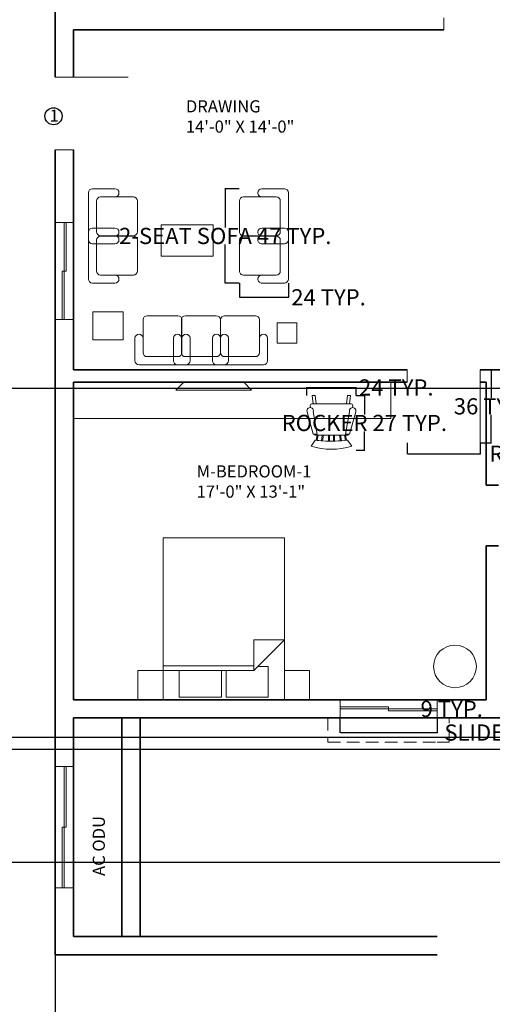
# Model space of a CAD drawing. Units: inches. Extents: x 3343 to 4790, y 1140 to 2641.
# Tile 7 of 10: x 4104 to 4337, y 1710 to 2196. Entities that reach past the tile are written whole.
import ezdxf

# ---------------------------------------------------------------- set-up
doc = ezdxf.new("R2010")
doc.units = ezdxf.units.IN
doc.header["$LTSCALE"] = 5
doc.header["$MEASUREMENT"] = 0
doc.linetypes.add('HIDDEN', pattern=[0.375, 0.25, -0.125])
for name, color, linetype, lineweight in [('A-ANNO-DIMS', 2, 'Continuous', 18), ('A-AREA-IDEN', 7, 'Continuous', 18), ('A-AREA-TAGS', 1, 'Continuous', 25), ('A-DOOR', 3, 'Continuous', 18), ('A-EQPM', 9, 'Continuous', 18), ('A-FLOR-CASE', 9, 'Continuous', 18), ('A-FLOR-HIDN', 8, 'HIDDEN', 13), ('A-FURN', 8, 'Continuous', 13), ('A-GLAZ', 4, 'Continuous', 18), ('A-WALL', 7, 'Continuous', 35)]:
    doc.layers.add(name, color=color, linetype=linetype, lineweight=lineweight)
doc.styles.get("Standard").update_dxf_attribs({"font": 'arial.ttf'})
doc.dimstyles.get("Standard").update_dxf_attribs({"dimtxt": 8, "dimasz": 0.18, "dimexe": 0.18, "dimexo": 0.0625, "dimgap": 0.09, "dimtad": 0, "dimtih": 1, "dimtoh": 1, "dimdec": 1, "dimzin": 0, "dimdsep": 46, "dimlunit": 3, "dimtxsty": 'Standard', "dimcen": 0.09, "dimadec": 0, "dimazin": 0, "dimtfac": 1, "dimtdec": 1, "dimtofl": 0, "dimtmove": 0, "dimatfit": 3, "dimfxl": 1, "dimtolj": 1, "dimtzin": 0, "dimarcsym": 0})

# ---------------------------------------------------------------- blocks, each defined once
blk = doc.blocks.new('Chair - Rocking')
for p, q in [((-8, -4.5), (-10, -1.5)), ((-7.5, -4.5), (-7, -7)), ((-6.5, -7), (-7.02225, -4.43)), ((-4.5, -7), (-4.96674, -4.19951)), ((-4, -7), (-4.40532, -4.16272)), ((-1.5, -4.05012), (-1.5, -7)), ((-1, -7), (-1, -4.05012)), ((1, -7), (1, -4.04655)), ((1.5, -4.05012), (1.5, -7)), ((4, -7), (4.40187, -4.18694)), ((4.5, -7), (4.96761, -4.19437)), ((6.5, -7), (7, -4.4057)), ((7.5, -4.5), (7, -7)), ((8, -4.5), (10, -1.5)), ((-9, -7.5), (-12, -18.49999)), ((-7, -7.5), (-9, -7.5)), ((-9, -18.49999), (-7, -7.5)), ((-8.23428, -6.99939), (-8.3093, -7.47958)), ((-8.23041, -7), (8.23915, -7)), ((7, -7.5), (9, -7.5)), ((9, -18.49999), (7, -7.5)), ((8.31071, -7.48854), (8.23449, -7.00073)), ((9, -7.5), (12, -18.49999)), ((-10.36644, -20.64523), (-10.5, -21.49999)), ((-9, -22.49999), (-9.5, -26.49999)), ((0, -22.49999), (-9.5, -22.49999)), ((-8, -26.49999), (-7.5, -22.49999)), ((0, -22.49999), (9.5, -22.49999)), ((8, -26.49999), (7.5, -22.49999)), ((9, -22.49999), (9.5, -26.49999)), ((10.5, -21.49999), (10.3575, -20.58798)), ((-9.5, -26.49999), (-8, -26.49999)), ((9.5, -26.49999), (8, -26.49999))]:
    blk.add_line(p, q)
for centre, radius, start, end in [((0, -34.08333), 34.08333, 72.93847, 107.0615), ((0, -68.25004), 64.25, 93.92211, 97.15267), ((0, -68.25004), 64.25, 82.84733, 93.92211), ((-10.5, -18.99999), 1.58114, 161.5651, 18.43495), ((10.5, -18.99999), 1.58114, 161.5651, 18.43495), ((-9.5, -21.49999), 1, 180, 270), ((9.5, -21.49999), 1, 270, 0)]:
    blk.add_arc(centre, radius, start, end)
blk = doc.blocks.new('Bed - Queen')
for p, q in [((0, -80.00003), (0, 0)), ((0, 0), (59.99999, 0)), ((59.99999, 0), (59.99999, -80.00003)), ((7.99999, -1.2), (28.79998, -1.2)), ((7.99999, -14.4), (7.99999, -1.2)), ((28.79998, -1.2), (28.79998, -14.4)), ((31.19999, -1.2), (51.99999, -1.2)), ((31.19999, -14.4), (31.19999, -1.2)), ((51.99999, -1.2), (51.99999, -16.4)), ((0, -14.4), (44.8, -14.4)), ((59.99999, -29.6), (44.8, -14.4)), ((44.8, -14.4), (44.8, -29.6)), ((44.8, -16.8), (0, -16.8)), ((51.99999, -16.4), (46.79936, -16.4)), ((44.8, -29.6), (59.99999, -29.6)), ((59.99999, -80.00003), (0, -80.00003))]:
    blk.add_line(p, q)
blk = doc.blocks.new('SOFA-2-SEAT')
for p, q in [((0, 22.22), (0, 11.11)), ((25.21, 24.22), (2, 24.22)), ((21.21, 20.22), (6, 20.22)), ((19.41, 22.22), (19.41, 11.11)), ((44.62, 24.22), (21.41, 24.22)), ((40.62, 20.22), (25.41, 20.22)), ((27.21, 11.11), (27.21, 22.22)), ((46.62, 11.11), (46.62, 22.22)), ((4, 18.22), (4, 11.11)), ((23.21, 11.11), (23.21, 18.22)), ((23.41, 18.22), (23.41, 11.11)), ((42.62, 11.11), (42.62, 18.22)), ((4, 11.11), (4, 2)), ((23.21, 11.11), (23.21, 2)), ((23.41, 11.11), (23.41, 2)), ((42.62, 11.11), (42.62, 2)), ((2, 9.11), (2, 9.11)), ((21.41, 9.11), (21.41, 9.11)), ((25.21, 9.11), (25.21, 9.11)), ((44.62, 9.11), (44.62, 9.11)), ((6, 0), (21.21, 0)), ((25.41, 0), (40.62, 0))]:
    blk.add_line(p, q)
for centre, start, end in [((2, 22.22), 90, 180), ((6, 18.22), 90, 180), ((21.41, 22.22), 90, 180), ((21.21, 18.22), 0, 90), ((25.41, 18.22), 90, 180), ((25.21, 22.22), 0, 90), ((40.62, 18.22), 0, 90), ((44.62, 22.22), 0, 90), ((2, 11.11), 180, 270), ((2, 11.11), 270, 0), ((21.41, 11.11), 180, 270), ((21.41, 11.11), 270, 0), ((25.21, 11.11), 180, 270), ((25.21, 11.11), 270, 0), ((44.62, 11.11), 180, 270), ((44.62, 11.11), 270, 0), ((6, 2), 180, 270), ((21.21, 2), 270, 0), ((25.41, 2), 180, 270), ((40.62, 2), 270, 0)]:
    blk.add_arc(centre, 2, start, end)
blk = doc.blocks.new('LOUNGE-CHAIR')
for p, q in [((4, 13.11), (4, 22.22)), ((6, 24.22), (21.21, 24.22)), ((23.21, 13.11), (23.21, 22.22)), ((2, 15.11), (2, 15.11)), ((25.21, 15.11), (25.21, 15.11)), ((0, 2), (0, 13.11)), ((4, 6), (4, 13.11)), ((23.21, 13.11), (23.21, 6)), ((27.21, 13.11), (27.21, 2)), ((21.21, 4), (6, 4)), ((25.21, 0), (2, 0))]:
    blk.add_line(p, q)
for centre, start, end in [((6, 22.22), 90, 180), ((21.21, 22.22), 0, 90), ((2, 13.11), 90, 180), ((2, 13.11), 0, 90), ((25.21, 13.11), 90, 180), ((25.21, 13.11), 0, 90), ((6, 6), 180, 270), ((21.21, 6), 270, 0), ((2, 2), 180, 270), ((25.21, 2), 270, 0)]:
    blk.add_arc(centre, 2, start, end)
blk = doc.blocks.new('TV-WALL-MOUNT')
for p, q in [((0, 37.4), (4.02, 33.55)), ((0, 0), (4.02, 3.86))]:
    blk.add_line(p, q)
for points in [[(0, 37.4), (0, 0)], [(4.02, 0), (4.02, 37.4)]]:
    blk.add_lwpolyline(points)
blk = doc.blocks.new('WINDOW-48IN-SLIDING-JAMB9')
for p, q in [((0, 9), (0, 0)), ((0, 5.5), (24, 5.5)), ((24, 5.5), (24, 3.5)), ((48, 9), (48, 0)), ((0, 4.5), (48, 4.5)), ((24, 3.5), (48, 3.5))]:
    blk.add_line(p, q)
blk = doc.blocks.new('WINDOW-60IN-SLIDING')
at = {"ltscale": 5}
for p, q in [((9, 60), (0, 60)), ((4.5, 60), (4.5, 0)), ((5.5, 60), (5.5, 30)), ((5.5, 30), (3.5, 30)), ((3.5, 30), (3.5, 0)), ((9, 0), (0, 0))]:
    blk.add_line(p, q, dxfattribs=at)
blk = doc.blocks.new('DOOR-36IN-6IN-JAMB')
for p, q in [((0, 30), (0, 36)), ((36, 30), (36, 36)), ((36, 36), (36, 0))]:
    blk.add_line(p, q)
blk = doc.blocks.new('NIGHTSTAND')
blk.add_lwpolyline([(12.43, 0), (0, 0), (0, 14.43), (12.43, 14.43)], close=True)
blk = doc.blocks.new('*D47')
at = {"layer": 'A-ANNO-DIMS', "color": 0, "lineweight": -2, "ltscale": 5, "transparency": 16777216}
for p, q in [((4261.87, 1851.1), (4261.87, 1843.78)), ((4309.87, 1851.1), (4309.87, 1843.78)), ((4262.05, 1843.96), (4309.69, 1843.96)), ((4309.87, 1843.96), (4310.05, 1843.96))]:
    blk.add_line(p, q, dxfattribs=at)
at = {"layer": 'A-ANNO-DIMS', "color": 0, "ltscale": 5, "transparency": 16777216}
for points in [[(4262.05, 1843.99), (4262.05, 1843.93), (4261.87, 1843.96)], [(4309.69, 1843.99), (4309.69, 1843.93), (4309.87, 1843.96)]]:
    blk.add_solid(points, dxfattribs=at)
at = {"layer": 'Defpoints', "color": 0, "ltscale": 5, "transparency": 16777216}
for p in [(4261.87, 1851.16), (4309.87, 1851.16), (4309.87, 1843.96)]:
    blk.add_point(p, dxfattribs=at)
at = {"layer": 'A-ANNO-DIMS', "color": 0, "ltscale": 5, "transparency": 16777216, "insert": (4351.33, 1843.96), "char_height": 8, "attachment_point": 5}
blk.add_mtext('\\A1;SLIDER 48 TYP.', dxfattribs=at)
blk = doc.blocks.new('*D48')
at = {"layer": 'A-ANNO-DIMS', "color": 0, "lineweight": -2, "ltscale": 5, "transparency": 16777216}
for p, q in [((4309.94, 1860.16), (4317.25, 1860.16)), ((4317.07, 1859.98), (4317.07, 1859.84)), ((4309.94, 1851.16), (4317.25, 1851.16)), ((4317.07, 1851.34), (4317.07, 1851.49))]:
    blk.add_line(p, q, dxfattribs=at)
at = {"layer": 'A-ANNO-DIMS', "color": 0, "ltscale": 5, "transparency": 16777216}
for points in [[(4317.04, 1859.98), (4317.1, 1859.98), (4317.07, 1860.16)], [(4317.04, 1851.34), (4317.1, 1851.34), (4317.07, 1851.16)]]:
    blk.add_solid(points, dxfattribs=at)
at = {"layer": 'Defpoints', "color": 0, "ltscale": 5, "transparency": 16777216}
for p in [(4309.87, 1860.16), (4317.07, 1860.16), (4309.87, 1851.16)]:
    blk.add_point(p, dxfattribs=at)
at = {"layer": 'A-ANNO-DIMS', "color": 0, "ltscale": 5, "transparency": 16777216, "insert": (4317.07, 1855.66), "char_height": 8, "attachment_point": 5}
blk.add_mtext('\\A1;9 TYP.', dxfattribs=at)
blk = doc.blocks.new('*D55')
at = {"layer": 'A-ANNO-DIMS', "color": 0, "lineweight": -2, "ltscale": 5, "transparency": 16777216}
for p, q in [((4269.92, 2010.44), (4274.09, 2010.44)), ((4273.91, 2010.26), (4273.91, 2001.17)), ((4273.91, 1983.62), (4273.91, 1992.71)), ((4269.92, 1983.44), (4274.09, 1983.44))]:
    blk.add_line(p, q, dxfattribs=at)
at = {"layer": 'A-ANNO-DIMS', "color": 0, "ltscale": 5, "transparency": 16777216}
for points in [[(4273.88, 2010.26), (4273.94, 2010.26), (4273.91, 2010.44)], [(4273.88, 1983.62), (4273.94, 1983.62), (4273.91, 1983.44)]]:
    blk.add_solid(points, dxfattribs=at)
at = {"layer": 'Defpoints', "color": 0, "ltscale": 5, "transparency": 16777216}
for p in [(4269.86, 2010.44), (4269.86, 1983.44), (4273.91, 1983.44)]:
    blk.add_point(p, dxfattribs=at)
at = {"layer": 'A-ANNO-DIMS', "color": 0, "ltscale": 5, "transparency": 16777216, "insert": (4273.91, 1996.94), "char_height": 8, "attachment_point": 5}
blk.add_mtext('\\A1;ROCKER 27 TYP.', dxfattribs=at)
blk = doc.blocks.new('*D56')
at = {"layer": 'A-ANNO-DIMS', "color": 0, "lineweight": -2, "ltscale": 5, "transparency": 16777216}
for p, q in [((4245.42, 2010.51), (4245.42, 2014.67)), ((4245.6, 2014.49), (4269.68, 2014.49)), ((4269.86, 2010.51), (4269.86, 2014.67)), ((4269.86, 2014.49), (4270.04, 2014.49))]:
    blk.add_line(p, q, dxfattribs=at)
at = {"layer": 'A-ANNO-DIMS', "color": 0, "ltscale": 5, "transparency": 16777216}
for points in [[(4245.6, 2014.52), (4245.6, 2014.46), (4245.42, 2014.49)], [(4269.68, 2014.52), (4269.68, 2014.46), (4269.86, 2014.49)]]:
    blk.add_solid(points, dxfattribs=at)
at = {"layer": 'Defpoints', "color": 0, "ltscale": 5, "transparency": 16777216}
for p in [(4269.86, 2014.49), (4245.42, 2010.44), (4269.86, 2010.44)]:
    blk.add_point(p, dxfattribs=at)
at = {"layer": 'A-ANNO-DIMS', "color": 0, "ltscale": 5, "transparency": 16777216, "insert": (4289.67, 2014.49), "char_height": 8, "attachment_point": 5}
blk.add_mtext('\\A1;24 TYP.', dxfattribs=at)
blk = doc.blocks.new('*D59')
at = {"layer": 'A-ANNO-DIMS', "color": 0, "lineweight": -2, "ltscale": 5, "transparency": 16777216}
for p, q in [((4212.1, 2112.65), (4204.99, 2112.65)), ((4205.17, 2112.47), (4205.17, 2093.57)), ((4205.17, 2066.22), (4205.17, 2085.12)), ((4212.1, 2066.04), (4204.99, 2066.04))]:
    blk.add_line(p, q, dxfattribs=at)
at = {"layer": 'A-ANNO-DIMS', "color": 0, "ltscale": 5, "transparency": 16777216}
for points in [[(4205.14, 2112.47), (4205.2, 2112.47), (4205.17, 2112.65)], [(4205.14, 2066.22), (4205.2, 2066.22), (4205.17, 2066.04)]]:
    blk.add_solid(points, dxfattribs=at)
at = {"layer": 'Defpoints', "color": 0, "ltscale": 5, "transparency": 16777216}
for p in [(4212.16, 2112.65), (4205.17, 2066.04), (4212.16, 2066.04)]:
    blk.add_point(p, dxfattribs=at)
at = {"layer": 'A-ANNO-DIMS', "color": 0, "ltscale": 5, "transparency": 16777216, "insert": (4205.17, 2089.34), "char_height": 8, "attachment_point": 5}
blk.add_mtext('\\A1;2-SEAT SOFA 47 TYP.', dxfattribs=at)
blk = doc.blocks.new('*D60')
at = {"layer": 'A-ANNO-DIMS', "color": 0, "lineweight": -2, "ltscale": 5, "transparency": 16777216}
for p, q in [((4212.16, 2065.97), (4212.16, 2058.86)), ((4236.39, 2065.97), (4236.39, 2058.86)), ((4212.34, 2059.04), (4236.21, 2059.04)), ((4236.39, 2059.04), (4236.57, 2059.04))]:
    blk.add_line(p, q, dxfattribs=at)
at = {"layer": 'A-ANNO-DIMS', "color": 0, "ltscale": 5, "transparency": 16777216}
for points in [[(4212.34, 2059.07), (4212.34, 2059.01), (4212.16, 2059.04)], [(4236.21, 2059.07), (4236.21, 2059.01), (4236.39, 2059.04)]]:
    blk.add_solid(points, dxfattribs=at)
at = {"layer": 'Defpoints', "color": 0, "ltscale": 5, "transparency": 16777216}
for p in [(4212.16, 2066.04), (4236.39, 2066.04), (4236.39, 2059.04)]:
    blk.add_point(p, dxfattribs=at)
at = {"layer": 'A-ANNO-DIMS', "color": 0, "ltscale": 5, "transparency": 16777216, "insert": (4256.2, 2059.04), "char_height": 8, "attachment_point": 5}
blk.add_mtext('\\A1;24 TYP.', dxfattribs=at)
blk = doc.blocks.new('*D63')
at = {"layer": 'A-ANNO-DIMS', "color": 0, "lineweight": -2, "ltscale": 5, "transparency": 16777216}
for p, q in [((4295.13, 1987.1), (4295.13, 1981.58)), ((4331.13, 1987.1), (4331.13, 1981.58)), ((4295.31, 1981.76), (4330.95, 1981.76)), ((4331.13, 1981.76), (4331.31, 1981.76))]:
    blk.add_line(p, q, dxfattribs=at)
at = {"layer": 'A-ANNO-DIMS', "color": 0, "ltscale": 5, "transparency": 16777216}
for points in [[(4295.31, 1981.79), (4295.31, 1981.73), (4295.13, 1981.76)], [(4330.95, 1981.79), (4330.95, 1981.73), (4331.13, 1981.76)]]:
    blk.add_solid(points, dxfattribs=at)
at = {"layer": 'Defpoints', "color": 0, "ltscale": 5, "transparency": 16777216}
for p in [(4295.13, 1987.16), (4331.13, 1987.16), (4331.13, 1981.76)]:
    blk.add_point(p, dxfattribs=at)
at = {"layer": 'A-ANNO-DIMS', "color": 0, "ltscale": 5, "transparency": 16777216, "insert": (4387.92, 1981.76), "char_height": 8, "attachment_point": 5}
blk.add_mtext('\\A1;ROOM DOOR 36 TYP.', dxfattribs=at)
blk = doc.blocks.new('*D64')
at = {"layer": 'A-ANNO-DIMS', "color": 0, "lineweight": -2, "ltscale": 5, "transparency": 16777216}
for p, q in [((4331.19, 2023.16), (4336.71, 2023.16)), ((4336.53, 2022.98), (4336.53, 2009.34)), ((4336.53, 1987.34), (4336.53, 2000.98)), ((4331.19, 1987.16), (4336.71, 1987.16))]:
    blk.add_line(p, q, dxfattribs=at)
at = {"layer": 'A-ANNO-DIMS', "color": 0, "ltscale": 5, "transparency": 16777216}
for points in [[(4336.5, 2022.98), (4336.56, 2022.98), (4336.53, 2023.16)], [(4336.5, 1987.34), (4336.56, 1987.34), (4336.53, 1987.16)]]:
    blk.add_solid(points, dxfattribs=at)
at = {"layer": 'Defpoints', "color": 0, "ltscale": 5, "transparency": 16777216}
for p in [(4331.13, 2023.16), (4336.53, 2023.16), (4331.13, 1987.16)]:
    blk.add_point(p, dxfattribs=at)
at = {"layer": 'A-ANNO-DIMS', "color": 0, "ltscale": 5, "transparency": 16777216, "insert": (4336.53, 2005.16), "char_height": 8, "attachment_point": 5}
blk.add_mtext('\\A1;36 TYP.', dxfattribs=at)
blk = doc.blocks.new('*D86')
at = {"layer": 'A-ANNO-DIMS', "color": 0, "lineweight": -2, "ltscale": 5, "transparency": 16777216}
for p, q in [((4121.13, 1851.1), (4121.13, 1144.78)), ((4674.13, 1851.1), (4674.13, 1144.78)), ((4121.31, 1144.96), (4388.7, 1144.96)), ((4673.95, 1144.96), (4406.56, 1144.96))]:
    blk.add_line(p, q, dxfattribs=at)
at = {"layer": 'A-ANNO-DIMS', "color": 0, "ltscale": 5, "transparency": 16777216}
for points in [[(4121.31, 1144.99), (4121.31, 1144.93), (4121.13, 1144.96)], [(4673.95, 1144.99), (4673.95, 1144.93), (4674.13, 1144.96)]]:
    blk.add_solid(points, dxfattribs=at)
at = {"layer": 'Defpoints', "color": 0, "ltscale": 5, "transparency": 16777216}
for p in [(4121.13, 1851.16), (4674.13, 1851.16), (4674.13, 1144.96)]:
    blk.add_point(p, dxfattribs=at)
at = {"layer": 'A-ANNO-DIMS', "color": 0, "ltscale": 5, "transparency": 16777216, "insert": (4397.63, 1144.96), "char_height": 8, "attachment_point": 5}
blk.add_mtext('\\A1;553', dxfattribs=at)
blk = doc.blocks.new('*D87')
at = {"layer": 'A-ANNO-DIMS', "color": 0, "lineweight": -2, "ltscale": 5, "transparency": 16777216}
for p, q in [((3977.19, 2566.16), (4773.46, 2566.16)), ((4773.28, 2565.98), (4773.28, 2294.34)), ((4773.28, 2014.34), (4773.28, 2285.99)), ((3977.19, 2014.16), (4773.46, 2014.16))]:
    blk.add_line(p, q, dxfattribs=at)
at = {"layer": 'A-ANNO-DIMS', "color": 0, "ltscale": 5, "transparency": 16777216}
for points in [[(4773.25, 2565.98), (4773.31, 2565.98), (4773.28, 2566.16)], [(4773.25, 2014.34), (4773.31, 2014.34), (4773.28, 2014.16)]]:
    blk.add_solid(points, dxfattribs=at)
at = {"layer": 'Defpoints', "color": 0, "ltscale": 5, "transparency": 16777216}
for p in [(3977.13, 2566.16), (3977.13, 2014.16), (4773.28, 2014.16)]:
    blk.add_point(p, dxfattribs=at)
at = {"layer": 'A-ANNO-DIMS', "color": 0, "ltscale": 5, "transparency": 16777216, "insert": (4773.28, 2290.16), "char_height": 8, "attachment_point": 5}
blk.add_mtext('\\A1;552', dxfattribs=at)
blk = doc.blocks.new('*D95')
at = {"layer": 'A-ANNO-DIMS', "color": 0, "lineweight": -2, "ltscale": 5, "transparency": 16777216}
for p, q in [((3637.31, 2014.16), (4773.46, 2014.16)), ((4773.28, 2013.98), (4773.28, 1932.09)), ((4773.28, 1841.85), (4773.28, 1923.74)), ((3610.31, 1841.67), (4773.46, 1841.67))]:
    blk.add_line(p, q, dxfattribs=at)
at = {"layer": 'A-ANNO-DIMS', "color": 0, "ltscale": 5, "transparency": 16777216}
for points in [[(4773.25, 2013.98), (4773.31, 2013.98), (4773.28, 2014.16)], [(4773.25, 1841.85), (4773.31, 1841.85), (4773.28, 1841.67)]]:
    blk.add_solid(points, dxfattribs=at)
at = {"layer": 'Defpoints', "color": 0, "ltscale": 5, "transparency": 16777216}
for p in [(3637.25, 2014.16), (3610.25, 1841.67), (4773.28, 1841.67)]:
    blk.add_point(p, dxfattribs=at)
at = {"layer": 'A-ANNO-DIMS', "color": 0, "ltscale": 5, "transparency": 16777216, "insert": (4773.28, 1927.92), "char_height": 8, "attachment_point": 5}
blk.add_mtext('\\A1;172.5', dxfattribs=at)
blk = doc.blocks.new('*D98')
at = {"layer": 'A-ANNO-DIMS', "color": 0, "lineweight": -2, "ltscale": 5, "transparency": 16777216}
for p, q in [((3811.31, 1835.67), (4773.46, 1835.67)), ((4773.28, 1835.49), (4773.28, 1811.94)), ((4773.28, 1780.04), (4773.28, 1803.59)), ((3811.31, 1779.86), (4773.46, 1779.86))]:
    blk.add_line(p, q, dxfattribs=at)
at = {"layer": 'A-ANNO-DIMS', "color": 0, "ltscale": 5, "transparency": 16777216}
for points in [[(4773.25, 1835.49), (4773.31, 1835.49), (4773.28, 1835.67)], [(4773.25, 1780.04), (4773.31, 1780.04), (4773.28, 1779.86)]]:
    blk.add_solid(points, dxfattribs=at)
at = {"layer": 'Defpoints', "color": 0, "ltscale": 5, "transparency": 16777216}
for p in [(3811.25, 1835.67), (3811.25, 1779.86), (4773.28, 1779.86)]:
    blk.add_point(p, dxfattribs=at)
at = {"layer": 'A-ANNO-DIMS', "color": 0, "ltscale": 5, "transparency": 16777216, "insert": (4773.28, 1807.76), "char_height": 8, "attachment_point": 5}
blk.add_mtext('\\A1;55.81', dxfattribs=at)

msp = doc.modelspace()

# ---------------------------------------------------------------- linework, layer by layer
at = {"layer": 'A-AREA-TAGS', "ltscale": 5}
msp.add_circle((4120.311, 2148.485), 4.235, dxfattribs=at)
at = {"layer": 'A-DOOR'}
for p, q in [((4130.13, 2167.871), (4121.13, 2167.871)), ((4121.13, 2167.871), (4157.13, 2167.871)), ((4130.13, 2131.871), (4121.13, 2131.871))]:
    msp.add_line(p, q, dxfattribs=at)
at = {"layer": 'A-FLOR-CASE'}
for p in [(4286.998, 2017.161), (4130.13, 1999.161)]:
    msp.add_line(p, (4286.998, 1999.161), dxfattribs=at)
at = {"layer": 'A-FLOR-HIDN', "ltscale": 5}
for p, q in [((4261.873, 1851.161), (4255.873, 1851.161)), ((4255.873, 1851.161), (4255.873, 1839.161)), ((4315.873, 1839.161), (4315.873, 1851.161)), ((4255.873, 1839.161), (4309.873, 1839.161)), ((4309.873, 1839.161), (4315.873, 1839.161)), ((4130.13, 1827.161), (4130.13, 1833.161))]:
    msp.add_line(p, q, dxfattribs=at)
at = {"layer": 'A-FURN'}
for points in [[(4173.526, 2094.806), (4199.219, 2094.806), (4199.219, 2079.38), (4173.526, 2079.38)], [(4139.722, 2051.833), (4154.78, 2051.833), (4154.78, 2037.978), (4139.722, 2037.978)], [(4230.831, 2046.345), (4240.55, 2046.345), (4240.55, 2036.292), (4230.831, 2036.292)]]:
    msp.add_lwpolyline(points, close=True, dxfattribs=at)
msp.add_circle((4318.692, 1876.644), 10.547, dxfattribs=at)
at = {"layer": 'A-WALL'}
for p, q in [((4121.13, 2441.161), (4121.13, 2167.871)), ((4130.13, 2191.161), (4313.13, 2191.161)), ((4130.13, 2191.161), (4130.13, 2167.871)), ((4121.13, 2131.871), (4121.13, 1851.161)), ((4130.13, 2131.871), (4130.13, 2023.161)), ((4130.13, 2023.161), (4295.13, 2023.161)), ((4331.13, 2023.161), (4452.13, 2023.161)), ((4130.13, 2017.161), (4295.13, 2017.161)), ((4130.13, 2017.161), (4130.13, 1860.161)), ((4331.13, 2017.161), (4334.13, 2017.161)), ((4334.13, 2017.161), (4334.13, 1966.161)), ((4340.13, 1966.161), (4334.13, 1966.161)), ((4340.13, 1936.161), (4334.13, 1936.161)), ((4334.13, 1936.161), (4334.13, 1860.161)), ((4130.13, 1860.161), (4334.13, 1860.161)), ((4130.13, 1851.161), (4309.873, 1851.161)), ((4154.13, 1743.161), (4154.13, 1851.161)), ((4163.13, 1743.161), (4163.13, 1851.161)), ((4309.873, 1851.161), (4545.72, 1851.161)), ((4130.13, 1743.161), (4309.873, 1743.161)), ((4121.13, 1734.161), (4309.873, 1734.161))]:
    msp.add_line(p, q, dxfattribs=at)
at = {"layer": 'A-WALL', "ltscale": 5}
for p, q in [((4121.13, 1851.161), (4121.13, 1734.161)), ((4130.13, 1851.161), (4130.13, 1743.161))]:
    msp.add_line(p, q, dxfattribs=at)

# ---------------------------------------------------------------- block references
at = {"layer": 'A-DOOR', "extrusion": (0, 0, -1), "zscale": -1, "rotation": 180}
msp.add_blockref('DOOR-36IN-6IN-JAMB', (-4313.13, 2227.161), dxfattribs=at)
at = {"layer": 'A-DOOR'}
msp.add_blockref('DOOR-36IN-6IN-JAMB', (4295.13, 1987.161), dxfattribs=at)
at = {"layer": 'A-EQPM', "rotation": 89.9999999999959}
msp.add_blockref('TV-WALL-MOUNT', (4218.182, 2013.142), dxfattribs=at)
at = {"layer": 'A-FURN'}
for p, rotation in [((4161.776, 2066.035), 89.99999999998057), ((4212.164, 2112.655), 270.0000000000143)]:
    msp.add_blockref('SOFA-2-SEAT', p, dxfattribs=dict(at, rotation=rotation))
for name, p in [('LOUNGE-CHAIR', (4160.56, 2025.695)), ('LOUNGE-CHAIR', (4179.545, 2025.695)), ('LOUNGE-CHAIR', (4198.862, 2025.695)), ('NIGHTSTAND', (4162.015, 1860.161)), ('NIGHTSTAND', (4234.443, 1860.161))]:
    msp.add_blockref(name, p, dxfattribs=at)
at = {"layer": 'A-FURN', "xscale": -1, "rotation": 180}
for name, p in [('Chair - Rocking', (4257.64, 1983.944)), ('Bed - Queen', (4174.443, 1860.161))]:
    msp.add_blockref(name, p, dxfattribs=at)
at = {"layer": 'A-GLAZ', "rotation": 269.9999999999977}
msp.add_blockref('WINDOW-48IN-SLIDING-JAMB9', (4121.13, 2095.991), dxfattribs=at)
at = {"layer": 'A-GLAZ'}
for name, p in [('WINDOW-48IN-SLIDING-JAMB9', (4261.873, 1851.161)), ('WINDOW-60IN-SLIDING', (4121.13, 1767.161))]:
    msp.add_blockref(name, p, dxfattribs=at)

# ---------------------------------------------------------------- texts
at = {"layer": 'A-AREA-IDEN', "ltscale": 5, "char_height": 6, "attachment_point": 1}
for s, insert in [('DRAWING\\P14\'-0" X 14\'-0"', (4185.73, 2156.389)), ('M-BEDROOM-1\\P17\'-0" X 13\'-1"', (4191.051, 1976.016))]:
    msp.add_mtext_dynamic_manual_height_columns(s, width=189.69543, gutter_width=1, heights=[0], dxfattribs=dict(at, insert=insert))
at = {"layer": 'A-AREA-IDEN', "ltscale": 5, "insert": (4139.692, 1773.092), "char_height": 6, "attachment_point": 1, "rotation": 90}
msp.add_mtext_dynamic_manual_height_columns('AC ODU', width=189.69543, gutter_width=1, heights=[0], dxfattribs=at)
at = {"layer": 'A-AREA-TAGS', "ltscale": 5, "insert": (4118.4, 2151.786), "char_height": 6, "attachment_point": 1}
msp.add_mtext_dynamic_manual_height_columns('1', width=189.69543, gutter_width=1, heights=[0], dxfattribs=at)

# ---------------------------------------------------------------- dimensions: what is measured, and where the dimension line sits
at = {"layer": 'A-ANNO-DIMS', "ltscale": 5}
for base, p1, p2, override, picture, middle in [((4773.28, 2014.161), (3977.13, 2566.161), (3977.13, 2014.161), {"dimdec": 0, "dimlfac": 1, "dimrnd": 0, "dimzin": 0, "dimdsep": 46, "dimlunit": 2}, '*D87', (4773.28, 2290.161)), ((4773.28, 1841.669), (3637.248, 2014.161), (3610.248, 1841.669), {"dimdec": 1, "dimlfac": 1, "dimrnd": 0, "dimzin": 0, "dimdsep": 46, "dimlunit": 2}, '*D95', (4773.28, 1927.915)), ((4773.28, 1779.857), (3811.248, 1835.669), (3811.248, 1779.857), {"dimdec": 2, "dimlfac": 1, "dimrnd": 0, "dimzin": 0, "dimdsep": 46, "dimlunit": 2}, '*D98', (4773.28, 1807.763))]:
    dim = msp.add_linear_dim(base=base, p1=p1, p2=p2, angle=90, dimstyle='Standard', override=override, dxfattribs=at)
    dim.commit()
    dim.dimension.update_dxf_attribs({"geometry": picture, "text_midpoint": middle})
for base, p1, p2, angle, text, picture, middle in [((4205.171, 2066.035), (4212.164, 2112.655), (4212.164, 2066.035), 270, '2-SEAT SOFA <> TYP.', '*D59', (4205.171, 2089.345)), ((4236.387, 2059.042), (4212.164, 2066.035), (4236.387, 2066.035), 0, '<> TYP.', '*D60', (4256.196, 2059.042)), ((4336.53, 2023.161), (4331.13, 1987.161), (4331.13, 2023.161), 90, '<> TYP.', '*D64', (4336.53, 2005.161)), ((4273.907, 1983.444), (4269.857, 2010.444), (4269.857, 1983.444), 270, 'ROCKER <> TYP.', '*D55', (4273.907, 1996.944)), ((4317.073, 1860.161), (4309.873, 1851.161), (4309.873, 1860.161), 90, '<> TYP.', '*D48', (4317.073, 1855.661))]:
    dim = msp.add_linear_dim(base=base, p1=p1, p2=p2, angle=angle, text=text, dimstyle='Standard', override={"dimdec": 0, "dimlfac": 1, "dimrnd": 0, "dimzin": 0, "dimdsep": 46, "dimlunit": 2}, dxfattribs=at)
    dim.commit()
    dim.dimension.update_dxf_attribs({"geometry": picture, "text_midpoint": middle})
for base, p1, p2, text, picture, middle in [((4269.857, 2014.494), (4245.422, 2010.444), (4269.857, 2010.444), '<> TYP.', '*D56', (4289.666, 2014.494)), ((4331.13, 1981.761), (4295.13, 1987.161), (4331.13, 1987.161), 'ROOM DOOR <> TYP.', '*D63', (4387.915, 1981.761)), ((4309.873, 1843.961), (4261.873, 1851.161), (4309.873, 1851.161), 'SLIDER <> TYP.', '*D47', (4351.333, 1843.961))]:
    dim = msp.add_linear_dim(base=base, p1=p1, p2=p2, text=text, dimstyle='Standard', override={"dimdec": 0, "dimlfac": 1, "dimrnd": 0, "dimzin": 0, "dimdsep": 46, "dimlunit": 2}, dxfattribs=at)
    dim.commit()
    dim.dimension.update_dxf_attribs({"geometry": picture, "text_midpoint": middle})
dim = msp.add_linear_dim(base=(4674.13, 1144.962), p1=(4121.13, 1851.161), p2=(4674.13, 1851.161), dimstyle='Standard', override={"dimdec": 0, "dimlfac": 1, "dimrnd": 0, "dimzin": 0, "dimdsep": 46, "dimlunit": 2}, dxfattribs=at)
dim.commit()
dim.dimension.update_dxf_attribs({"geometry": '*D86', "text_midpoint": (4397.63, 1144.962)})

doc.saveas('drawing.dxf')
